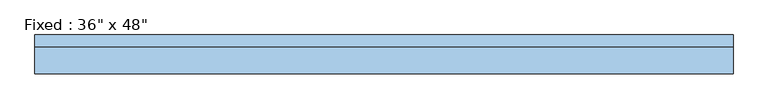
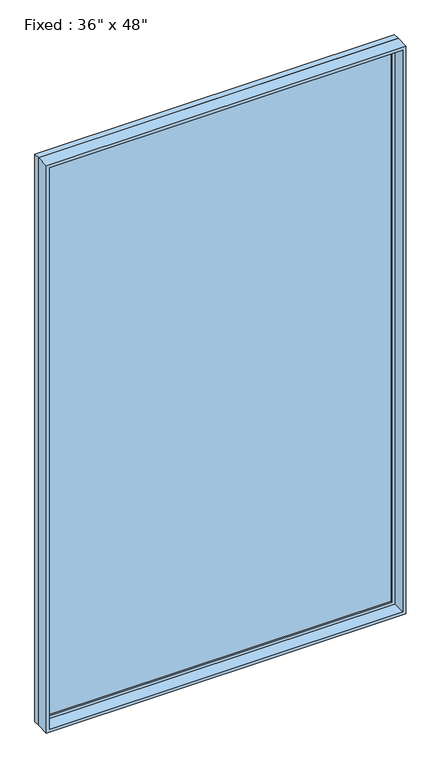
"""IFC4 building model written with IfcOpenShell, lengths in millimetres: window geometry."""

from ifc_helpers import new_model, si_unit, frame, origin, place, context, project, spatial, polyline, outline, extrude, source, transform, mapped, element, save


def window_c349b51b(model_context):
    return source(origin(), model_context, "Body", "SweptSolid", [
        extrude(outline(polyline([(1727.2, 53.975), (-1803.4, 53.975), (-1803.4, 66.675), (1727.2, 66.675), (1727.2, 53.975)])), frame((0.0, 0.0, 977.9), z_axis=(0.0, 0.0, 1.0), x_axis=(1.0, 0.0, 0.0)), (0.0, 0.0, 1.0), 5969.0),
        extrude(outline(polyline([(6991.35, -1847.85), (933.45, -1847.85), (933.45, 1771.65), (6991.35, 1771.65), (6991.35, -1847.85)]), holes=[polyline([(6946.9, -1803.4), (6946.9, 1727.2), (977.9, 1727.2), (977.9, -1803.4), (6946.9, -1803.4)])]), frame((0.0, 38.1, 0.0), z_axis=(0.0, 1.0, 0.0), x_axis=(0.0, 0.0, 1.0)), (0.0, 0.0, 1.0), 44.45),
        extrude(outline(polyline([(7010.4, -1866.9), (914.4, -1866.9), (914.4, 1790.7), (7010.4, 1790.7), (7010.4, -1866.9)]), holes=[polyline([(6978.65, -1835.15), (6978.65, 1758.95), (946.15, 1758.95), (946.15, -1835.15), (6978.65, -1835.15)])]), frame((0.0, -101.6, 0.0), z_axis=(0.0, 1.0, 0.0), x_axis=(0.0, 0.0, 1.0)), (0.0, 0.0, 1.0), 139.7),
        extrude(outline(polyline([(7010.4, 1790.7), (7010.4, -1866.9), (914.4, -1866.9), (914.4, 1790.7), (7010.4, 1790.7)]), holes=[polyline([(6991.35, 1771.65), (933.45, 1771.65), (933.45, -1847.85), (6991.35, -1847.85), (6991.35, 1771.65)])]), frame((0.0, 38.1, 0.0), z_axis=(0.0, 1.0, 0.0), x_axis=(0.0, 0.0, 1.0)), (0.0, 0.0, 1.0), 63.5),
    ])


if __name__ == "__main__":
    model = new_model("IFC4")
    model_context = context("Model", 3, world=origin())
    ifc_project = project(units=[si_unit("LENGTHUNIT", "METRE", prefix="MILLI")], contexts=[model_context])
    site = spatial("IfcSite", under=ifc_project)
    building = spatial("IfcBuilding", under=site)
    placement = place(None, origin())
    window_shape = window_c349b51b(model_context)
    element("IfcWindow", 1, ObjectType="Fixed : 36\" x 48\"", at=placement, inside=building, context=model_context, shape_type="MappedRepresentation", body=[
        mapped(window_shape, transform((0.0, 0.0, 0.0), x_axis=(1.0, 0.0, 0.0), y_axis=(0.0, 1.0, 0.0), z_axis=(0.0, 0.0, 1.0))),
    ])
    save(model, "model.ifc")

# Revit data of these elements
# Type "Fixed : 36\" x 48\""
#   Type Mark = "1"
#   Construction Type Id = "GSP4R"
#   Assembly Code = "B2020100"
#   Analytic Construction = "1/8 in Pilkington single glazing"
#   Visual Light Transmittance = 0.9
#   Solar Heat Gain Coefficient = 0.78
#   Heat Transfer Coefficient (U) = 0.6496 BTU/(h·ft²·°F)
#   Height = 20' - 0"
#   Default Sill Height = 3' - 0"
#   Width = 12' - 0"
#   Window Inset = 0' - 0 3/4"
#   Define Thermal Properties by = 1
#   Glass Pane Material = Glass
#   Sash Material = Sash
#   Wall Closure = (empty or 0)
# Element 1 (IfcWindow, "Fixed : 36\" x 48\"")
#   Materials on its faces: "Sash", "Glass"
# Materials
#   "Glass": class "Glass", colour RGB 0 128 192, transparency 0.75, Description = "Soda Lime Glass", Cost = 0
#   "Sash": class "Wood", colour RGB 224 178 126, transparency 0
